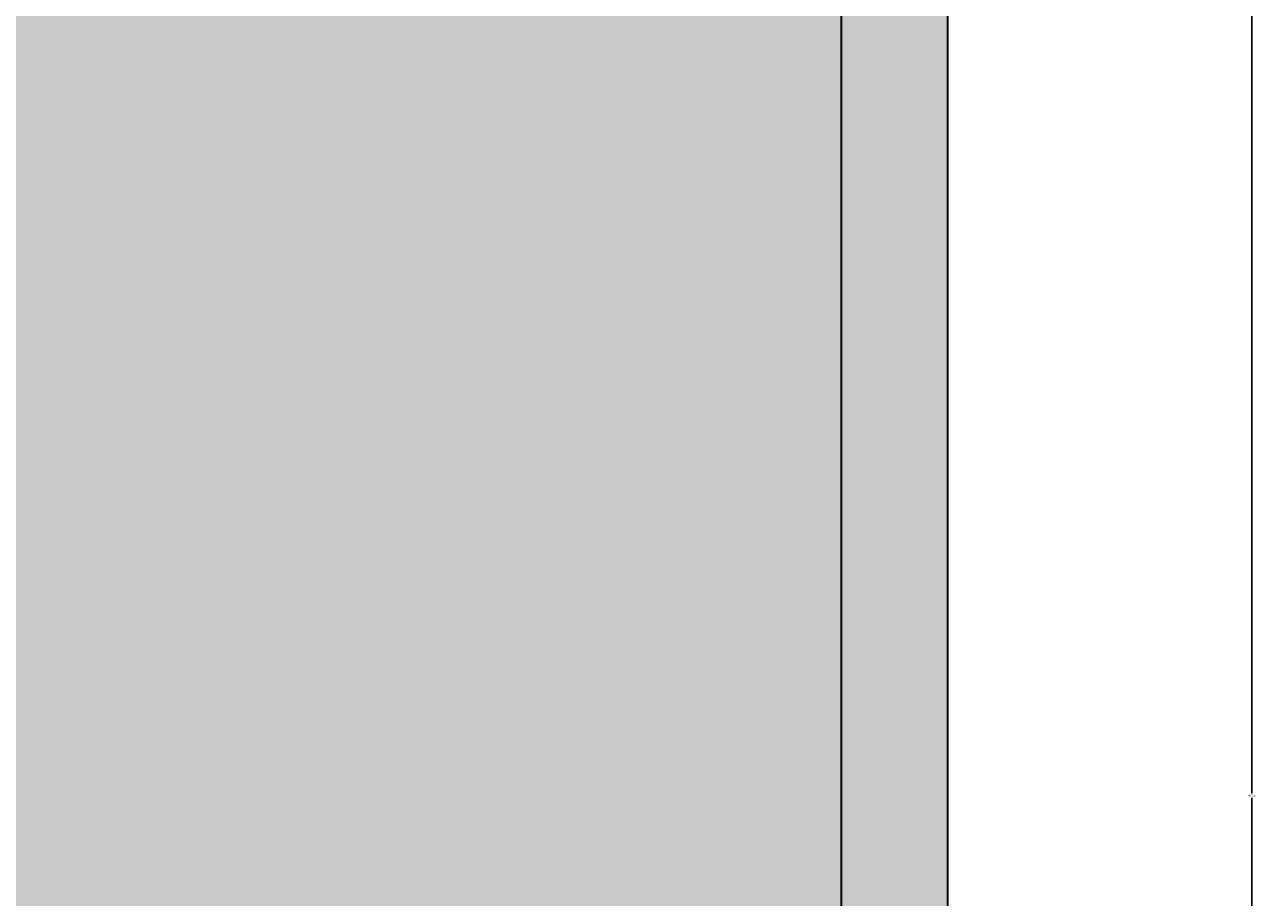
# Model space of a CAD drawing. Units: inches. Extents: x 3024 to 3952, y 1308 to 1863.
# Tile 21 of 29: x 3392 to 3496, y 1559 to 1633. Entities that reach past the tile are written whole.
import ezdxf

# ---------------------------------------------------------------- set-up
doc = ezdxf.new("R2010")
doc.units = ezdxf.units.IN
for name, color, linetype, lineweight in [('A-ANNO-DIMS', 2, 'Continuous', 18), ('A-FLOR-TILE-PATT', 7, 'Continuous', 13), ('A-WALL', 7, 'Continuous', 35)]:
    doc.layers.add(name, color=color, linetype=linetype, lineweight=lineweight)
doc.layers.add('A-FLOR-PATT', color=254, linetype='Continuous', lineweight=13, true_color=0xfeeab9)
doc.layers.add('A-WALL-PATT', color=254, linetype='Continuous', lineweight=13, true_color=0xcecce6)
doc.styles.get("Standard").update_dxf_attribs({"font": 'arial.ttf'})
doc.dimstyles.get("Standard").update_dxf_attribs({"dimtxt": 0.18, "dimasz": 0.18, "dimexe": 0.18, "dimexo": 0.0625, "dimgap": 0.09, "dimtad": 0, "dimtih": 1, "dimtoh": 1, "dimdec": 4, "dimzin": 0, "dimdsep": 46, "dimtxsty": 'Standard', "dimcen": 0.09, "dimadec": 0, "dimazin": 0, "dimtfac": 1, "dimtdec": 4, "dimtofl": 0, "dimtmove": 0, "dimatfit": 3, "dimfxl": 1, "dimtolj": 1, "dimtzin": 0, "dimarcsym": 0})

# ---------------------------------------------------------------- blocks, each defined once
blk = doc.blocks.new('*D37')
at = {"layer": 'A-ANNO-DIMS', "color": 0, "lineweight": -2, "transparency": 16777216}
for p, q in [((3469.83, 1787.61), (3495.72, 1787.61)), ((3495.54, 1787.43), (3495.54, 1567.91)), ((3495.54, 1348.03), (3495.54, 1567.54)), ((3469.83, 1347.85), (3495.72, 1347.85))]:
    blk.add_line(p, q, dxfattribs=at)
at = {"layer": 'A-ANNO-DIMS', "color": 0, "transparency": 16777216}
for points in [[(3495.51, 1787.43), (3495.57, 1787.43), (3495.54, 1787.61)], [(3495.51, 1348.03), (3495.57, 1348.03), (3495.54, 1347.85)]]:
    blk.add_solid(points, dxfattribs=at)
at = {"layer": 'Defpoints', "color": 0, "transparency": 16777216}
for p in [(3469.76, 1787.61), (3495.54, 1787.61), (3469.76, 1347.85)]:
    blk.add_point(p, dxfattribs=at)
at = {"layer": 'A-ANNO-DIMS', "color": 0, "transparency": 16777216, "insert": (3495.54, 1567.73), "char_height": 0.18, "attachment_point": 5}
blk.add_mtext('\\A1;439.8', dxfattribs=at)

msp = doc.modelspace()

# ---------------------------------------------------------------- hatches: boundary and pattern name
at = {"layer": 'A-FLOR-PATT', "transparency": 33554528}
h = msp.add_hatch(color=256, dxfattribs=at)
h.dxf.hatch_style = 1
h.paths.add_polyline_path([(3460.764, 1688.6064), (3412.764, 1688.6064), (3412.764, 1694.6064), (3460.764, 1694.6064), (3460.764, 1778.6064), (3406.764, 1778.6064), (3406.764, 1759.9514), (3318.2981, 1759.9514), (3318.2981, 1658.6064), (3322.5356, 1658.6064), (3322.5356, 1652.6064), (3292.764, 1652.6064), (3292.764, 1778.6064), (3106.764, 1778.6064), (3106.764, 1628.6064), (3172.764, 1628.6064), (3172.764, 1532.6064), (3166.764, 1532.6064), (3166.764, 1628.6064), (3106.764, 1628.6064), (3106.764, 1356.8452), (3202.812, 1356.8452), (3202.812, 1354.2534), (3202.812, 1353.8388), (3202.812, 1351.1212), (3202.812, 1347.8452), (3277.764, 1347.8452), (3277.764, 1353.8452), (3277.764, 1356.8452), (3277.764, 1442.6064), (3460.764, 1442.6064)])
h.paths.add_polyline_path([(3216.238, 1527.2064), (3216.238, 1491.2064), (3214.663, 1491.2064), (3214.663, 1491.2409, -0.39662236), (3180.243, 1526.6064), (3163.0285, 1526.6064), (3163.0285, 1531.1064), (3161.716, 1531.1064), (3161.716, 1561.1064), (3163.0285, 1561.1064), (3163.0285, 1531.1064), (3163.0285, 1526.6064), (3180.243, 1526.6064, 0.39662236), (3214.663, 1491.2409), (3214.663, 1527.2064)], flags=16)
h.paths.add_polyline_path([(3227.364, 1649.8972), (3191.364, 1649.8972), (3191.364, 1651.4722), (3227.364, 1651.4722)], flags=16)
h.paths.add_polyline_path([(3323.1172, 1606.7362), (3323.8545, 1606.8514), (3323.8545, 1594.8241), (3323.1172, 1594.9393)], flags=16)
h.paths.add_polyline_path([(3324.2232, 1606.909), (3330.1216, 1607.8307), (3330.1216, 1614.1093), (3339.3495, 1614.1093), (3340.2711, 1620.0078), (3352.4136, 1620.0078), (3353.3353, 1614.1093), (3359.9941, 1614.1093), (3360.9157, 1620.0078), (3373.0582, 1620.0078), (3373.9799, 1614.1093), (3383.2077, 1614.1093), (3383.2077, 1607.8307), (3389.1062, 1606.909), (3389.1062, 1594.7665), (3383.2077, 1593.8449), (3383.2077, 1587.5663), (3373.9799, 1587.5663), (3373.0583, 1581.6678), (3360.9157, 1581.6678), (3359.9941, 1587.5663), (3353.3353, 1587.5663), (3352.4136, 1581.6678), (3340.2711, 1581.6678), (3339.3495, 1587.5663), (3330.1216, 1587.5663), (3330.1216, 1593.8449), (3324.2232, 1594.7665)], flags=16)
h.paths.add_polyline_path([(3236.1584, 1693.1064), (3236.1584, 1723.1064), (3237.4709, 1723.1064), (3237.4709, 1693.1064)], flags=16)
h.paths.add_polyline_path([(3373.2158, 1600.6847), (3373.7965, 1600.7303), (3374.3268, 1600.7874), (3374.8132, 1600.8531), (3375.2621, 1600.9247), (3375.6801, 1600.9991), (3376.0736, 1601.0735), (3376.6855, 1601.19), (3377.366, 1601.3023), (3378.0667, 1601.3814), (3378.8026, 1601.4123), (3379.5865, 1601.3839), (3380.4537, 1601.2948), (3381.301, 1601.1717), (3382.0317, 1601.0433), (3382.4398, 1600.9607), (3382.6252, 1600.9201), (3382.919, 1600.8507), (3382.9044, 1600.8531), (3382.842, 1600.8678), (3382.7541, 1600.8896), (3382.6252, 1600.9201), (3382.4398, 1600.9607), (3382.1868, 1601.0119), (3381.8738, 1601.0711), (3381.5125, 1601.1346), (3381.1149, 1601.1988), (3380.6928, 1601.2601), (3380.2581, 1601.3149), (3379.8226, 1601.3597), (3379.3984, 1601.3908), (3378.9944, 1601.4054), (3378.6092, 1601.4042), (3378.2384, 1601.3886), (3377.8777, 1601.36), (3377.5227, 1601.32), (3377.1691, 1601.2698), (3376.8127, 1601.211), (3376.4491, 1601.145), (3376.0736, 1601.0735), (3375.4177, 1600.9494), (3374.5542, 1600.8119), (3373.5044, 1600.6988)], flags=0)
h.paths.add_polyline_path([(3380.0253, 1596.7351), (3380.499, 1596.6659), (3380.9706, 1596.6119), (3381.4375, 1596.5791), (3381.8971, 1596.5736), (3382.5886, 1596.6167), (3382.7848, 1596.6692), (3382.1465, 1596.5706), (3381.236, 1596.5815), (3380.3199, 1596.6865)], flags=0)
h.paths.add_polyline_path([(3369.6414, 1603.9617), (3370.1589, 1604.0021), (3370.6218, 1604.0539), (3371.0335, 1604.1173), (3371.3978, 1604.1921), (3371.7181, 1604.2785), (3371.9984, 1604.3761), (3372.2441, 1604.483), (3372.4611, 1604.5972), (3372.655, 1604.7163), (3372.8317, 1604.8384), (3372.9968, 1604.9611), (3373.3703, 1605.2455), (3373.8426, 1605.5328), (3374.4624, 1605.7539), (3375.1058, 1605.8302), (3375.7221, 1605.8261), (3376.4109, 1605.76), (3377.1534, 1605.6376), (3377.8945, 1605.473), (3378.1382, 1605.409), (3377.7394, 1605.5074), (3377.3509, 1605.5937), (3376.9704, 1605.6677), (3376.5999, 1605.7288), (3376.2417, 1605.7762), (3375.8979, 1605.8092), (3375.5707, 1605.8271), (3375.2621, 1605.8291), (3374.9745, 1605.8146), (3374.7092, 1605.7832), (3374.4647, 1605.7359), (3374.239, 1605.6742), (3374.0298, 1605.5996), (3373.835, 1605.5134), (3373.6525, 1605.4171), (3373.4801, 1605.3123), (3373.3156, 1605.2002), (3373.1562, 1605.0825), (3372.7603, 1604.781), (3372.236, 1604.4588), (3371.5738, 1604.2283), (3370.8493, 1604.0794), (3369.9262, 1603.976)], flags=0)
h.paths.add_polyline_path([(3366.7533, 1606.5832), (3367.1713, 1606.5519), (3367.5378, 1606.5374), (3367.8568, 1606.5394), (3368.1325, 1606.5573), (3368.3694, 1606.5903), (3368.5717, 1606.6377), (3368.7438, 1606.6988), (3368.89, 1606.7728), (3369.0146, 1606.8591), (3369.121, 1606.9568), (3369.2094, 1607.0646), (3369.2792, 1607.181), (3369.3295, 1607.3046), (3369.3596, 1607.4339), (3369.3688, 1607.5676), (3369.3565, 1607.7042), (3369.3218, 1607.8422), (3369.2649, 1607.9804), (3369.1893, 1608.1187), (3369.0993, 1608.2569), (3368.9992, 1608.3952), (3368.8934, 1608.5334), (3368.7861, 1608.6717), (3368.6817, 1608.8099), (3368.4212, 1609.1804), (3368.2685, 1609.7106), (3368.4883, 1610.1814), (3369.0537, 1610.4604), (3369.6717, 1610.5097), (3370.2812, 1610.3612), (3370.4805, 1610.2968), (3370.1882, 1610.3839), (3369.9284, 1610.4472), (3369.6905, 1610.4842), (3369.4662, 1610.4933), (3369.2555, 1610.4765), (3369.0608, 1610.4367), (3368.884, 1610.3767), (3368.7274, 1610.2994), (3368.5931, 1610.2077), (3368.4833, 1610.1045), (3368.4002, 1609.9927), (3368.3451, 1609.8747), (3368.3166, 1609.7517), (3368.3127, 1609.6244), (3368.331, 1609.4935), (3368.3696, 1609.3597), (3368.4261, 1609.2237), (3368.4985, 1609.0863), (3368.5845, 1608.9482), (3368.6817, 1608.8099), (3368.7861, 1608.6717), (3368.8934, 1608.5334), (3368.9992, 1608.3952), (3369.0993, 1608.2569), (3369.3398, 1607.8876), (3369.3941, 1607.2896), (3368.9774, 1606.7817), (3368.3928, 1606.5742), (3367.7162, 1606.5303), (3367.0044, 1606.5585)], flags=0)
h.paths.add_polyline_path([(3362.1859, 1610.2589), (3362.5478, 1610.2845), (3362.8348, 1610.3275), (3363.0585, 1610.3863), (3363.2303, 1610.4595), (3363.3619, 1610.5457), (3363.463, 1610.6432), (3363.5376, 1610.7502), (3363.5876, 1610.8643), (3363.6153, 1610.9834), (3363.6229, 1611.1055), (3363.6125, 1611.2283), (3363.5861, 1611.3496), (3363.5462, 1611.4673), (3363.4949, 1611.5797), (3363.4358, 1611.6871), (3363.3723, 1611.7902), (3363.3081, 1611.8897), (3363.2468, 1611.9863), (3363.192, 1612.0808), (3363.0258, 1612.4261), (3363.3371, 1612.8672), (3363.9008, 1612.9782), (3364.4822, 1612.9641), (3365.1098, 1612.9074), (3365.328, 1612.8805), (3364.9615, 1612.9208), (3364.6426, 1612.9496), (3364.3668, 1612.9669), (3364.1299, 1612.9726), (3363.9276, 1612.9669), (3363.7555, 1612.9496), (3363.6093, 1612.9208), (3363.4848, 1612.8805), (3363.3782, 1612.8289), (3363.2889, 1612.7672), (3363.2169, 1612.6969), (3363.1622, 1612.6193), (3363.1247, 1612.5361), (3363.1046, 1612.4484), (3363.1017, 1612.358), (3363.1161, 1612.266), (3363.1472, 1612.1738), (3363.192, 1612.0808), (3363.2468, 1611.9863), (3363.3081, 1611.8897), (3363.3723, 1611.7902), (3363.4358, 1611.6871), (3363.6363, 1611.323), (3363.5979, 1610.7003), (3363.0863, 1610.3651), (3362.3983, 1610.2622)], flags=0)
h.paths.add_polyline_path([(3352.356, 1581.2991), (3352.2408, 1580.5618), (3340.4439, 1580.5618), (3340.3287, 1581.2991)], flags=16)
h.paths.add_polyline_path([(3340.4439, 1621.1137), (3352.2408, 1621.1137), (3352.356, 1620.3764), (3340.3287, 1620.3764)], flags=16)
h.paths.add_polyline_path([(3278.4282, 1504.7424), (3290.3831, 1504.7424), (3290.3831, 1502.7499), (3291.0473, 1502.7499), (3291.0473, 1494.7799), (3290.3831, 1494.7799), (3290.3831, 1494.1158), (3291.0473, 1494.1158), (3291.0473, 1486.1458), (3290.3831, 1486.1458), (3290.3831, 1484.1533), (3291.0473, 1484.1533), (3291.0473, 1483.4892, -0.09090909), (3291.0473, 1468.8776), (3291.0473, 1468.2135), (3290.3831, 1468.2135), (3290.3831, 1464.8926), (3278.4282, 1464.8926), (3278.4282, 1472.8626), (3277.764, 1473.5268), (3277.764, 1478.84), (3278.4282, 1479.5042)], flags=16)
h.paths.add_polyline_path([(3278.7603, 1504.4103), (3290.051, 1504.4103), (3290.051, 1465.2247), (3278.7603, 1465.2247)], flags=0)
h.paths.add_polyline_path([(3123.904, 1600.7821), (3117.9039, 1602.7821), (3117.9039, 1599.7821), (3119.4039, 1599.7821), (3119.4039, 1596.7821), (3118.4039, 1596.7821), (3118.4039, 1598.7821), (3117.9039, 1598.7821), (3117.9039, 1596.2821), (3109.9039, 1596.2821), (3109.9039, 1617.2821), (3117.9039, 1617.2821), (3117.9039, 1610.7821), (3123.9038, 1612.7821, -0.70257121), (3137.9039, 1606.7822, -0.70256205)], flags=16)
h.paths.add_polyline_path([(3123.9039, 1602.7822), (3123.9039, 1610.7822, -0.73453329), (3136.9039, 1606.7822, -0.73452973)], flags=0)
h.paths.add_polyline_path([(3177.972, 1689.6473), (3109.2405, 1689.6473), (3109.2405, 1741.1959), (3177.972, 1741.1959)], flags=16)
h.paths.add_polyline_path([(3373.0006, 1581.2991), (3372.8854, 1580.5618), (3361.0885, 1580.5618), (3360.9733, 1581.2991)], flags=16)
h.paths.add_polyline_path([(3361.0885, 1621.1137), (3372.8854, 1621.1137), (3373.0006, 1620.3764), (3360.9733, 1620.3764)], flags=16)
h.paths.add_polyline_path([(3116.9039, 1598.2821, -0.41421356), (3116.1539, 1597.2821), (3111.9039, 1597.2821, -0.41421356), (3110.9039, 1598.0321), (3110.9039, 1615.2821, -0.41421356), (3111.6539, 1616.2821), (3115.9039, 1616.2821, -0.41421356), (3116.9039, 1615.5321)], flags=0)
h.paths.add_polyline_path([(3121.6122, 1728.1369), (3121.6122, 1696.5205), (3110.2715, 1696.5205), (3110.2715, 1714.3906), (3121.6122, 1714.3906), (3121.6122, 1716.4526), (3110.2715, 1716.4526), (3110.2715, 1734.3228), (3123.3304, 1734.3228), (3123.3304, 1729.8552), (3134.6711, 1741.1959), (3134.6711, 1728.1369)], flags=0)
h.paths.add_polyline_path([(3389.4748, 1606.8514), (3390.2122, 1606.7362), (3390.2122, 1594.9393), (3389.4748, 1594.8241)], flags=16)
h.paths.add_polyline_path([(3257.6842, 1762.8281), (3259.6842, 1768.8281), (3256.6842, 1768.8281), (3256.6842, 1767.3281), (3253.6842, 1767.3281), (3253.6842, 1768.3281), (3255.6842, 1768.3281), (3255.6842, 1768.8281), (3253.1842, 1768.8281), (3253.1842, 1776.8281), (3274.1842, 1776.8281), (3274.1842, 1768.8281), (3267.6842, 1768.8281), (3269.6842, 1762.8282, -0.70257121), (3263.6843, 1748.8282, -0.70256205)], flags=16)
h.paths.add_polyline_path([(3259.6842, 1762.8281), (3267.6843, 1762.8281, -0.73453329), (3263.6842, 1749.8282, -0.73452973)], flags=0)
h.paths.add_polyline_path([(3411.264, 1715.6064), (3411.264, 1716.9189), (3441.264, 1716.9189), (3441.264, 1715.6064)], flags=16)
h.paths.add_polyline_path([(3178.3806, 1449.1876), (3178.3806, 1397.639), (3109.6491, 1397.639), (3109.6491, 1449.1876)], flags=16)
h.paths.add_polyline_path([(3397.1501, 1541.7146), (3419.6183, 1541.7146), (3419.6183, 1496.7783), (3397.1501, 1496.7783)], flags=16)
h.paths.add_polyline_path([(3254.1842, 1770.5781), (3254.1842, 1774.8281, -0.41421356), (3254.9342, 1775.8281), (3272.1842, 1775.8281, -0.41421356), (3273.1842, 1775.0781), (3273.1842, 1770.8281, -0.41421356), (3272.4342, 1769.8281), (3255.1842, 1769.8281, -0.41421356)], flags=0)
h.paths.add_polyline_path([(3403.672, 1500.7601), (3403.6016, 1500.3997), (3403.5328, 1500.0441), (3403.4662, 1499.6867), (3403.4027, 1499.3226), (3403.3464, 1498.9532), (3403.3025, 1498.5811), (3403.2759, 1498.2091), (3403.2714, 1497.8401), (3403.3064, 1497.2813), (3403.3491, 1497.1219), (3403.2689, 1497.6395), (3403.2778, 1498.3719), (3403.3635, 1499.0984), (3403.4889, 1499.8168), (3403.6016, 1500.3997), (3403.672, 1500.7601), (3403.744, 1501.1315), (3403.817, 1501.5205), (3403.891, 1501.9336), (3403.9656, 1502.3769), (3404.0404, 1502.8572), (3404.115, 1503.3786), (3404.2264, 1504.2311), (3404.2571, 1504.5223), (3404.1552, 1503.6598), (3404.0063, 1502.6193), (3403.8604, 1501.7518), (3403.744, 1501.1315)], flags=0)
h.paths.add_polyline_path([(3406.5868, 1505.0416), (3406.6121, 1504.5236), (3406.6492, 1504.0526), (3406.6956, 1503.624), (3406.7491, 1503.2333), (3406.8072, 1502.8759), (3406.8676, 1502.5473), (3406.9281, 1502.243), (3407.0268, 1501.7597), (3407.1416, 1501.1368), (3407.2087, 1500.3904), (3407.1804, 1499.6703), (3407.1078, 1498.9956), (3407.0074, 1498.3199), (3406.8809, 1497.6059), (3406.7403, 1496.9627), (3406.7418, 1496.9824), (3406.7491, 1497.0249), (3406.8229, 1497.3409), (3406.8364, 1497.4025), (3406.878, 1497.6078), (3406.9261, 1497.8614), (3406.9777, 1498.1526), (3407.0298, 1498.4712), (3407.0797, 1498.8068), (3407.1243, 1499.149), (3407.1607, 1499.4874), (3407.1859, 1499.8115), (3407.1978, 1500.1137), (3407.1969, 1500.3962), (3407.1841, 1500.6642), (3407.1609, 1500.9225), (3407.1284, 1501.1761), (3407.0876, 1501.43), (3407.0398, 1501.6891), (3406.9862, 1501.9585), (3406.8832, 1502.4628), (3406.7712, 1503.0713), (3406.6657, 1503.8424), (3406.5924, 1504.7735)], flags=0)
h.paths.add_polyline_path([(3409.2517, 1507.8962), (3409.2752, 1507.4282), (3409.3079, 1507.0076), (3409.3501, 1506.6314), (3409.4015, 1506.2969), (3409.4624, 1506.0009), (3409.5326, 1505.7406), (3409.6119, 1505.5128), (3409.6988, 1505.3131), (3409.7915, 1505.1368), (3409.8883, 1504.9792), (3409.9875, 1504.8356), (3410.0872, 1504.7015), (3410.1859, 1504.572), (3410.4508, 1504.2132), (3410.7205, 1503.6035), (3410.8059, 1502.8824), (3410.7619, 1502.0875), (3410.6122, 1501.2299), (3410.4402, 1500.6169), (3410.2538, 1500.0031), (3410.0536, 1499.3219), (3409.9909, 1499.0812), (3410.1761, 1499.7472), (3410.3596, 1500.3513), (3410.4512, 1500.6561), (3410.5312, 1500.9412), (3410.6013, 1501.226), (3410.6614, 1501.512), (3410.7111, 1501.7964), (3410.7496, 1502.0763), (3410.7764, 1502.3489), (3410.7909, 1502.6114), (3410.7926, 1502.8608), (3410.7808, 1503.0944), (3410.7553, 1503.31), (3410.7169, 1503.5087), (3410.6667, 1503.6921), (3410.6061, 1503.8621), (3410.5361, 1504.0203), (3410.4578, 1504.1686), (3410.3726, 1504.3088), (3410.2815, 1504.4424), (3410.1859, 1504.572), (3410.0872, 1504.7015), (3409.859, 1505.0083), (3409.5943, 1505.5117), (3409.4266, 1506.1336), (3409.324, 1506.8011), (3409.2586, 1507.6407)], flags=0)
h.paths.add_polyline_path([(3411.4914, 1510.5878), (3411.4432, 1510.1586), (3411.4054, 1509.775), (3411.38, 1509.4354), (3411.3681, 1509.1376), (3411.3698, 1508.8784), (3411.3843, 1508.6542), (3411.4112, 1508.4618), (3411.4497, 1508.2974), (3411.4994, 1508.1575), (3411.5595, 1508.0388), (3411.6296, 1507.9375), (3411.7097, 1507.851), (3411.802, 1507.7792), (3411.9096, 1507.7225), (3412.0353, 1507.6817), (3412.1821, 1507.6572), (3412.3528, 1507.6496), (3412.5505, 1507.6597), (3412.778, 1507.6879), (3413.0364, 1507.7341), (3413.3194, 1507.7955), (3413.6188, 1507.8687), (3413.9264, 1507.95), (3414.234, 1508.036), (3414.5333, 1508.1232), (3414.8163, 1508.208), (3415.0747, 1508.287), (3415.3023, 1508.3569), (3415.5007, 1508.4158), (3415.6733, 1508.4617), (3416.1158, 1508.5538), (3416.512, 1508.2591), (3416.716, 1507.6581), (3416.61, 1507.0003), (3416.3052, 1506.3411), (3415.8928, 1505.618), (3415.7339, 1505.3633), (3415.9914, 1505.791), (3416.201, 1506.1583), (3416.3666, 1506.4739), (3416.4925, 1506.7462), (3416.5828, 1506.9838), (3416.6413, 1507.1949), (3416.6725, 1507.3883), (3416.6799, 1507.5705), (3416.6662, 1507.7417), (3416.6339, 1507.9), (3416.5851, 1508.0436), (3416.5223, 1508.1709), (3416.4478, 1508.28), (3416.3639, 1508.3692), (3416.273, 1508.4368), (3416.1765, 1508.4815), (3416.0718, 1508.5047), (3415.9553, 1508.5079), (3415.8237, 1508.493), (3415.6733, 1508.4617), (3415.5007, 1508.4158), (3415.3327, 1508.3659), (3414.6495, 1508.157), (3414.0606, 1507.9855), (3413.4456, 1507.8229), (3412.8838, 1507.701), (3412.5505, 1507.6597), (3412.0748, 1507.6354), (3411.595, 1507.8883), (3411.398, 1508.4429), (3411.3624, 1508.9927), (3411.3854, 1509.5711), (3411.4578, 1510.3071)], flags=0)
h.paths.add_polyline_path([(3135.0797, 1449.1876), (3135.0797, 1436.1286), (3122.0208, 1436.1286), (3122.0208, 1404.5122), (3110.6801, 1404.5122), (3110.6801, 1422.3823), (3122.0208, 1422.3823), (3122.0208, 1424.4443), (3110.6801, 1424.4443), (3110.6801, 1442.3145), (3123.739, 1442.3145), (3123.739, 1437.8469)], flags=0)
h.paths.add_polyline_path([(3416.4944, 1514.2949), (3416.4837, 1513.8511), (3416.4893, 1513.4867), (3416.5102, 1513.1926), (3416.5451, 1512.9593), (3416.5929, 1512.7775), (3416.6524, 1512.6379), (3416.7224, 1512.531), (3416.8017, 1512.4488), (3416.8886, 1512.3882), (3416.9813, 1512.3476), (3417.0781, 1512.3251), (3417.1773, 1512.3189), (3417.277, 1512.3274), (3417.3757, 1512.3488), (3417.4713, 1512.3813), (3417.5627, 1512.4229), (3417.65, 1512.471), (3417.7338, 1512.5225), (3417.8146, 1512.5747), (3417.8931, 1512.6245), (3417.9699, 1512.6691), (3418.2968, 1512.8265), (3418.6505, 1512.4645), (3418.7037, 1511.9342), (3418.6693, 1511.3839), (3418.6076, 1510.8228), (3418.5777, 1510.5927), (3418.6197, 1510.9333), (3418.6525, 1511.2311), (3418.6759, 1511.4903), (3418.6899, 1511.7144), (3418.6946, 1511.9069), (3418.6899, 1512.0713), (3418.6759, 1512.2112), (3418.6525, 1512.33), (3418.6197, 1512.4311), (3418.5778, 1512.5177), (3418.5276, 1512.5903), (3418.4705, 1512.6488), (3418.4075, 1512.6933), (3418.3399, 1512.7237), (3418.2686, 1512.7401), (3418.1951, 1512.7424), (3418.1204, 1512.7307), (3418.0455, 1512.7055), (3417.9792, 1512.6736), (3417.65, 1512.471), (3417.5627, 1512.4229), (3417.4713, 1512.3813), (3417.3757, 1512.3488), (3417.277, 1512.3274), (3416.878, 1512.2936), (3416.5757, 1512.7549), (3416.492, 1513.3145), (3416.4808, 1514.0384)], flags=0)
h.paths.add_polyline_path([(3392.8223, 1481.9454), (3396.7707, 1481.9454), (3396.7707, 1480.9201), (3428.3585, 1480.9201), (3428.3585, 1481.9454), (3432.3069, 1481.9454), (3432.3069, 1464.8354, -0.26666697), (3392.8223, 1464.8354)], flags=16)
h.paths.add_polyline_path([(3431.203, 1547.5428), (3450.8613, 1547.5428, -0.19047621), (3450.8614, 1484.031), (3431.203, 1484.031), (3431.203, 1488.5675), (3432.3809, 1488.5675), (3432.3809, 1543.0062), (3431.203, 1543.0062)], flags=16)
h.paths.add_polyline_path([(3451.9233, 1524.86, -0.04962821), (3451.9233, 1506.7138), (3446.7921, 1506.7138), (3446.7921, 1524.86)], flags=0)
h.paths.add_polyline_path([(3460.764, 1436.6064), (3277.764, 1436.6064), (3277.764, 1356.8452), (3277.764, 1353.8452), (3460.764, 1353.8452)], flags=17)
h.paths.add_polyline_path([(3121.3033, 1577.378), (3153.693, 1577.378), (3153.693, 1586.6752), (3121.3033, 1586.6752)], flags=24)
h.paths.add_polyline_path([(3164.1457, 1464.1276), (3210.4801, 1464.1276), (3210.4801, 1473.4247), (3164.1457, 1473.4247)], flags=24)
h.paths.add_polyline_path([(3343.1909, 1505.8863), (3373.7236, 1505.8863), (3373.7236, 1515.1773), (3343.1909, 1515.1773)], flags=24)
h.paths.add_polyline_path([(3337.6353, 1564.2926), (3370.0189, 1564.2926), (3370.0189, 1573.5836), (3337.6353, 1573.5836)], flags=24)
h.paths.add_polyline_path([(3419.204, 1753.8578), (3453.3997, 1753.8578), (3453.3997, 1762.9956), (3419.204, 1762.9956)], flags=24)
h.paths.add_polyline_path([(3341.2523, 1701.0246), (3381.0761, 1701.0246), (3381.0761, 1710.3156), (3341.2523, 1710.3156)], flags=24)
h.paths.add_polyline_path([(3245.8895, 1726.2997), (3278.2793, 1726.2997), (3278.2793, 1735.5968), (3245.8895, 1735.5968)], flags=24)
h.paths.add_polyline_path([(3128.8045, 1668.6736), (3175.1389, 1668.6736), (3175.1389, 1677.9707), (3128.8045, 1677.9707)], flags=24)
h.paths.add_polyline_path([(3345.9997, 1396.0062), (3389.09, 1396.0062), (3389.09, 1405.3033), (3345.9997, 1405.3033)], flags=24)
at = {"layer": 'A-FLOR-TILE-PATT', "transparency": 33554569}
h = msp.add_hatch(dxfattribs=at)
h.set_pattern_fill('ANGLE', color=256, scale=2)
h.set_pattern_definition([(0, (0, 0), (0, 13.97), [10.16, -3.81]), (90, (0, 0), (-13.97, 9e-16), [10.16, -3.81])])
h.paths.add_polyline_path([(3292.764, 1778.6064), (3232.764, 1778.6064), (3232.764, 1694.6064), (3236.1584, 1694.6064), (3236.1584, 1723.1064), (3237.4709, 1723.1064), (3237.4709, 1723.0777, -0.38700389), (3266.1209, 1694.6064), (3292.764, 1694.6064)])
h.paths.add_polyline_path([(3263.6843, 1748.8282, -0.70256205), (3257.6842, 1762.8281), (3259.6842, 1768.8281), (3256.6842, 1768.8281), (3256.6842, 1767.3281), (3253.6842, 1767.3281), (3253.6842, 1768.3281), (3255.6842, 1768.3281), (3255.6842, 1768.8281), (3253.1842, 1768.8281), (3253.1842, 1776.8281), (3274.1842, 1776.8281), (3274.1842, 1768.8281), (3267.6842, 1768.8281), (3269.6842, 1762.8282, -0.70257121)], flags=16)
h.paths.add_polyline_path([(3263.6842, 1749.8282, -0.73452973), (3259.6842, 1762.8281), (3267.6843, 1762.8281, -0.73453329)], flags=0)
h.paths.add_polyline_path([(3255.1842, 1769.8281, -0.41421356), (3254.1842, 1770.5781), (3254.1842, 1774.8281, -0.41421356), (3254.9342, 1775.8281), (3272.1842, 1775.8281, -0.41421356), (3273.1842, 1775.0781), (3273.1842, 1770.8281, -0.41421356), (3272.4342, 1769.8281)], flags=0)
h.paths.add_polyline_path([(3460.764, 1436.6064), (3277.764, 1436.6064), (3277.764, 1356.8452), (3277.764, 1353.8452), (3460.764, 1353.8452)])
h.paths.add_polyline_path([(3166.764, 1628.6064), (3106.764, 1628.6064), (3106.764, 1532.6064), (3133.066, 1532.6064, -0.38700389), (3161.716, 1561.0777), (3161.716, 1561.1064), (3163.0285, 1561.1064), (3163.0285, 1532.6064), (3166.764, 1532.6064)])
h.paths.add_polyline_path([(3123.904, 1600.7821), (3117.9039, 1602.7821), (3117.9039, 1599.7821), (3119.4039, 1599.7821), (3119.4039, 1596.7821), (3118.4039, 1596.7821), (3118.4039, 1598.7821), (3117.9039, 1598.7821), (3117.9039, 1596.2821), (3109.9039, 1596.2821), (3109.9039, 1617.2821), (3117.9039, 1617.2821), (3117.9039, 1610.7821), (3123.9038, 1612.7821, -0.70257121), (3137.9039, 1606.7822, -0.70256205)], flags=16)
h.paths.add_polyline_path([(3123.9039, 1602.7822), (3123.9039, 1610.7822, -0.73453329), (3136.9039, 1606.7822, -0.73452973)], flags=0)
h.paths.add_polyline_path([(3116.1539, 1597.2821), (3111.9039, 1597.2821, -0.41421356), (3110.9039, 1598.0321), (3110.9039, 1615.2821, -0.41421356), (3111.6539, 1616.2821), (3115.9039, 1616.2821, -0.41421356), (3116.9039, 1615.5321), (3116.9039, 1598.2821, -0.41421356)], flags=0)
h.paths.add_polyline_path([(3245.8895, 1726.2997), (3278.2793, 1726.2997), (3278.2793, 1735.5968), (3245.8895, 1735.5968)], flags=24)
h.paths.add_polyline_path([(3345.9997, 1396.0062), (3389.09, 1396.0062), (3389.09, 1405.3033), (3345.9997, 1405.3033)], flags=24)
h.paths.add_polyline_path([(3121.3033, 1577.378), (3153.693, 1577.378), (3153.693, 1586.6752), (3121.3033, 1586.6752)], flags=24)
at = {"layer": 'A-WALL-PATT'}
h = msp.add_hatch(color=256, dxfattribs=at)
h.dxf.hatch_style = 1
h.paths.add_polyline_path([(3106.764, 1778.6064), (3140.5977, 1778.6064), (3140.5977, 1781.8824), (3140.5977, 1784.6), (3140.5977, 1787.6064), (3097.764, 1787.6064), (3097.764, 1590.213), (3101.04, 1590.213), (3103.7576, 1590.213), (3106.764, 1590.213)])
h.paths.add_polyline_path([(3253.5314, 1781.8824), (3253.5314, 1784.6), (3253.5314, 1787.6064), (3194.6826, 1787.6064), (3194.6826, 1785.0146), (3194.6826, 1784.6), (3194.6826, 1781.8824), (3194.6826, 1778.6064), (3253.5314, 1778.6064)])
h.paths.add_polyline_path([(3333.856, 1782.2838), (3333.856, 1784.7474), (3333.856, 1787.6064), (3272.0523, 1787.6064), (3272.0523, 1785.0146), (3272.0523, 1784.6), (3272.0523, 1781.8824), (3272.0523, 1778.6064), (3333.856, 1778.6064)])
h.paths.add_polyline_path([(3428.8344, 1784.6), (3428.8344, 1787.6064), (3378.3947, 1787.6064), (3378.3947, 1784.7474), (3378.3947, 1782.2838), (3378.3947, 1778.6064), (3428.8344, 1778.6064), (3428.8344, 1781.8824)], flags=17)
h.paths.add_polyline_path([(3469.764, 1787.6064), (3451.9386, 1787.6064), (3451.9386, 1785.0146), (3451.9386, 1784.6), (3451.9386, 1781.8824), (3451.9386, 1778.6064), (3460.764, 1778.6064), (3460.764, 1353.8452), (3277.764, 1353.8452), (3277.764, 1347.8452), (3469.764, 1347.8452), (3469.764, 1353.8452)])
h.paths.add_polyline_path([(3106.764, 1571.6922), (3104.1722, 1571.6922), (3103.7576, 1571.6922), (3101.04, 1571.6922), (3097.764, 1571.6922), (3097.764, 1347.8452), (3148.7271, 1347.8452), (3148.7271, 1351.1212), (3148.7271, 1353.8388), (3148.7271, 1356.8452), (3106.764, 1356.8452)])
h.paths.add_polyline_path([(3277.764, 1532.6064), (3262.7605, 1532.6064), (3262.7605, 1582.9359), (3256.7605, 1582.9359), (3256.7605, 1532.6064), (3244.2116, 1532.6064), (3216.238, 1532.6064), (3216.238, 1527.2064), (3216.238, 1526.6064), (3271.764, 1526.6064), (3271.764, 1356.8452), (3202.812, 1356.8452), (3202.812, 1354.2534), (3202.812, 1353.8388), (3202.812, 1351.1212), (3202.812, 1347.8452), (3277.764, 1347.8452), (3277.764, 1353.8452), (3277.764, 1356.8452)])
h.paths.add_polyline_path([(3180.238, 1532.6064), (3163.0285, 1532.6064), (3163.0285, 1531.1064), (3163.0285, 1526.6064), (3180.243, 1526.6064, -0.00416688), (3180.238, 1527.2064)])
h.paths.add_polyline_path([(3133.0285, 1531.1064, -0.01250587), (3133.066, 1532.6064), (3106.764, 1532.6064), (3106.764, 1526.6064), (3133.0285, 1526.6064)], flags=17)
h.paths.add_polyline_path([(3172.764, 1628.6064), (3166.764, 1628.6064), (3166.764, 1532.6064), (3172.764, 1532.6064)])
h.paths.add_polyline_path([(3232.764, 1649.8972), (3227.364, 1649.8972), (3226.764, 1649.8972), (3226.764, 1634.6064), (3106.764, 1634.6064), (3106.764, 1628.6064), (3232.764, 1628.6064)])

# ---------------------------------------------------------------- linework, layer by layer
at = {"layer": 'A-WALL'}
for p, q in [((3469.764, 1347.8452), (3469.764, 1787.6064)), ((3460.764, 1353.8452), (3460.764, 1778.6064))]:
    msp.add_line(p, q, dxfattribs=at)

# ---------------------------------------------------------------- dimensions: what is measured, and where the dimension line sits
at = {"layer": 'A-ANNO-DIMS'}
dim = msp.add_linear_dim(base=(3495.539, 1787.6064), p1=(3469.764, 1347.8452), p2=(3469.764, 1787.6064), angle=90, dimstyle='Standard', override={"dimdec": 1, "dimlfac": 1, "dimrnd": 0, "dimzin": 0, "dimdsep": 46, "dimlunit": 2}, dxfattribs=at)
dim.commit()
dim.dimension.update_dxf_attribs({"geometry": '*D37', "text_midpoint": (3495.539, 1567.7258)})

doc.saveas('drawing.dxf')
